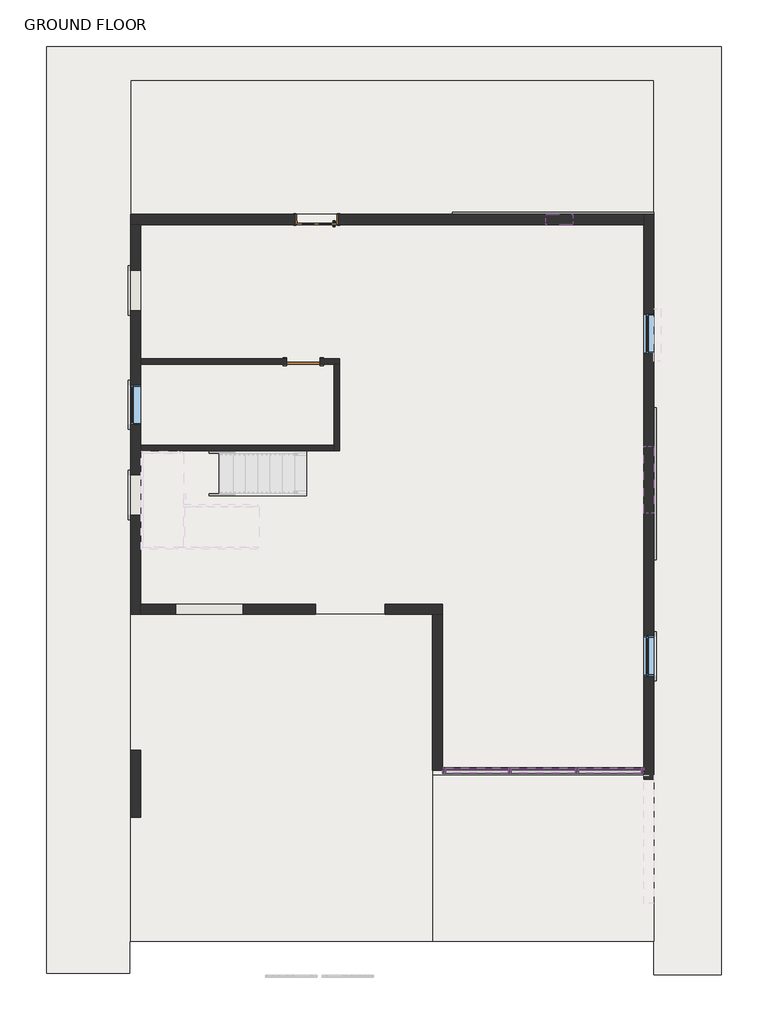
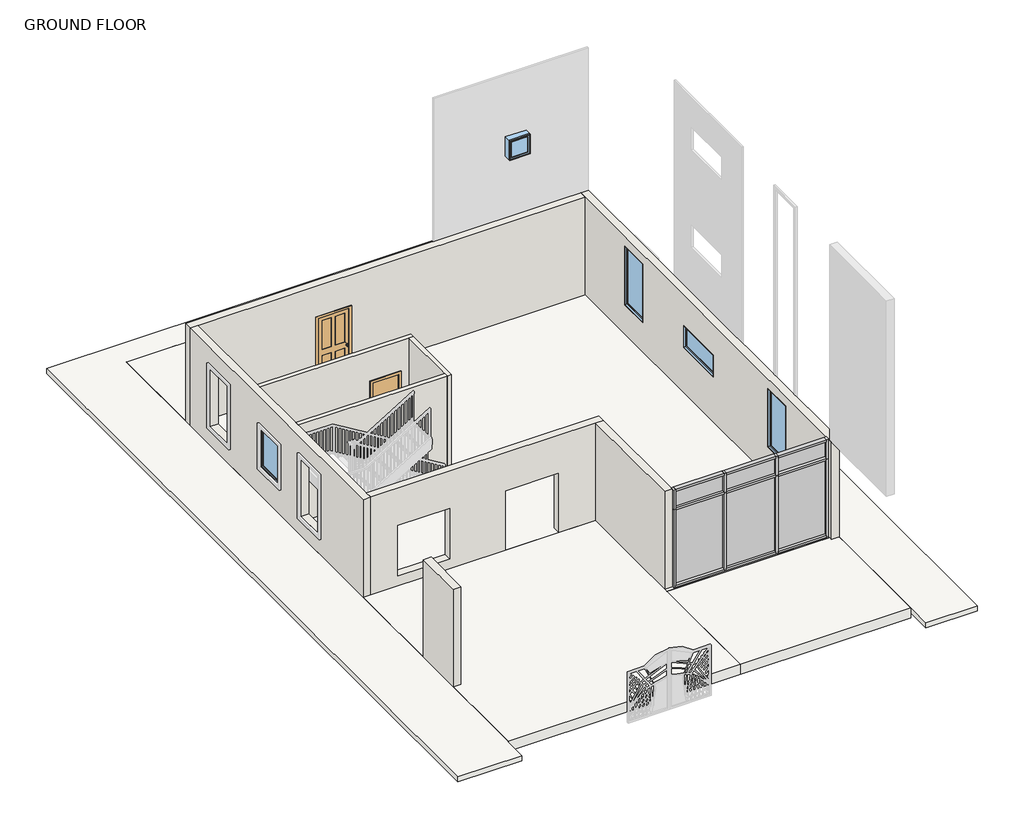
# One storey, part 1 of 3: 17 members, 9 walls, 6 plates, 5 slabs, 5 windows, 2 doors.
"""IFC4 building model written with IfcOpenShell, lengths in millimetres."""

from ifc_helpers import new_model, si_unit, frame, origin, origin_with_axes, place, context, project, spatial, polyline, outline, extrude, faceted_brep, transform, mapped, element, save
from components import door_8a5afc22, door_1fe7f57d, member_f0fea5a5, member_ee409385, member_3473b942, member_19b327e1, member_2e265c97, member_a95d9ad3, member_6e77e263, member_47bfaf8a, system_panel_glazed_f9f53b74, system_panel_glazed_d986c6a7, system_panel_glazed_28169b10, system_panel_glazed_6dc8f8fc, window_80340324, window_c1f32544, window_2e8ca8a3, window_e88f44c6

model = new_model("IFC4")

# Units and contexts
model_context = context("Model", 3, world=origin())
ifc_project = project(units=[si_unit("LENGTHUNIT", "METRE", prefix="MILLI")], contexts=[model_context])

# Site, building, storey
site = spatial("IfcSite", under=ifc_project)
building = spatial("IfcBuilding", under=site)
storey = spatial("IfcBuildingStorey", under=building, Name="GROUND FLOOR", Elevation=304.8)

# Doors
placement = place(None, origin())
door_shape = door_8a5afc22(model_context)
element("IfcDoor", 1, ObjectType="Door-Interior-Single-4_Panel-Wood : 36\" x 80\"", at=placement, inside=storey, context=model_context, shape_type="MappedRepresentation", body=[
    mapped(door_shape, transform((-5763.4781265, 8218.7107468, 304.8), x_axis=(-1.0, 0.0, 0.0), y_axis=(0.0, -1.0, 0.0), z_axis=(0.0, 0.0, 1.0))),
])
door_2_shape = door_1fe7f57d(model_context)
element("IfcDoor", 2, ObjectType="Single-Flush : 30\" x 80\"", at=placement, inside=storey, context=model_context, shape_type="MappedRepresentation", body=[
    mapped(door_2_shape, transform((-6068.2781265, 4996.0857468, 304.8), x_axis=(-1.0, 0.0, 0.0), y_axis=(0.0, -1.0, 0.0), z_axis=(0.0, 0.0, 1.0))),
])

# Members
member_shape = member_f0fea5a5(model_context)
element("IfcMember", 3, ObjectType="Rectangular Mullion : 2.5\" x 5\" rectangular", at=placement, inside=storey, context=model_context, shape_type="MappedRepresentation", body=[
    mapped(member_shape, transform((-1381.9781264, -4274.9142532, 304.8), x_axis=(1.0, 0.0, 0.0), y_axis=(0.0, -1.0, 0.0), z_axis=(0.0, 0.0, -1.0))),
])
element("IfcMember", 4, ObjectType="Rectangular Mullion : 2.5\" x 5\" rectangular", at=placement, inside=storey, context=model_context, shape_type="MappedRepresentation", body=[
    mapped(member_shape, transform((142.0218734, -4274.9142532, 304.8), x_axis=(1.0, 0.0, 0.0), y_axis=(0.0, -1.0, 0.0), z_axis=(0.0, 0.0, -1.0))),
])
member_2_shape = member_ee409385(model_context)
element("IfcMember", 5, ObjectType="Rectangular Mullion : 2.5\" x 5\" rectangular", at=placement, inside=storey, context=model_context, shape_type="MappedRepresentation", body=[
    mapped(member_2_shape, transform((1666.0218735, -4274.9142532, 304.8), x_axis=(1.0, 0.0, 0.0), y_axis=(0.0, -1.0, 0.0), z_axis=(0.0, 0.0, -1.0))),
])
element("IfcMember", 6, ObjectType="Rectangular Mullion : 2.5\" x 5\" rectangular", at=placement, inside=storey, context=model_context, shape_type="MappedRepresentation", body=[
    mapped(member_2_shape, transform((-2905.9781265, -4274.9142532, 2743.2), x_axis=(-1.0, 0.0, 0.0), y_axis=(0.0, -1.0, 0.0), z_axis=(0.0, 0.0, 1.0))),
])
member_3_shape = member_3473b942(model_context)
element("IfcMember", 7, ObjectType="Rectangular Mullion : 2.5\" x 5\" rectangular", at=placement, inside=storey, context=model_context, shape_type="MappedRepresentation", body=[
    mapped(member_3_shape, transform((1602.5218735, -4274.9142532, 3352.8), x_axis=(0.0, 0.0, 1.0), y_axis=(0.0, -1.0, 0.0), z_axis=(1.0, 0.0, 0.0))),
])
element("IfcMember", 8, ObjectType="Rectangular Mullion : 2.5\" x 5\" rectangular", at=placement, inside=storey, context=model_context, shape_type="MappedRepresentation", body=[
    mapped(member_3_shape, transform((-1413.7281264, -4274.9142532, 3352.8), x_axis=(0.0, 0.0, 1.0), y_axis=(0.0, -1.0, 0.0), z_axis=(1.0, 0.0, 0.0))),
])
element("IfcMember", 9, ObjectType="Rectangular Mullion : 2.5\" x 5\" rectangular", at=placement, inside=storey, context=model_context, shape_type="MappedRepresentation", body=[
    mapped(member_3_shape, transform((-2842.4781265, -4274.9142532, 304.8), x_axis=(0.0, 0.0, -1.0), y_axis=(0.0, -1.0, 0.0), z_axis=(-1.0, 0.0, 0.0))),
])
element("IfcMember", 10, ObjectType="Rectangular Mullion : 2.5\" x 5\" rectangular", at=placement, inside=storey, context=model_context, shape_type="MappedRepresentation", body=[
    mapped(member_3_shape, transform((173.7718734, -4274.9142532, 304.8), x_axis=(0.0, 0.0, -1.0), y_axis=(0.0, -1.0, 0.0), z_axis=(-1.0, 0.0, 0.0))),
])
member_4_shape = member_19b327e1(model_context)
element("IfcMember", 11, ObjectType="Rectangular Mullion : 2.5\" x 5\" rectangular", at=placement, inside=storey, context=model_context, shape_type="MappedRepresentation", body=[
    mapped(member_4_shape, transform((110.2718734, -4274.9142532, 3352.8), x_axis=(0.0, 0.0, 1.0), y_axis=(0.0, -1.0, 0.0), z_axis=(1.0, 0.0, 0.0))),
])
element("IfcMember", 12, ObjectType="Rectangular Mullion : 2.5\" x 5\" rectangular", at=placement, inside=storey, context=model_context, shape_type="MappedRepresentation", body=[
    mapped(member_4_shape, transform((-1350.2281264, -4274.9142532, 304.8), x_axis=(0.0, 0.0, -1.0), y_axis=(0.0, -1.0, 0.0), z_axis=(-1.0, 0.0, 0.0))),
])
member_5_shape = member_2e265c97(model_context)
element("IfcMember", 13, ObjectType="Rectangular Mullion : 2.5\" x 5\" rectangular", at=placement, inside=storey, context=model_context, shape_type="MappedRepresentation", body=[
    mapped(member_5_shape, transform((-1413.7281264, -4274.9142532, 2743.2), x_axis=(0.0, 0.0, 1.0), y_axis=(0.0, -1.0, 0.0), z_axis=(1.0, 0.0, 0.0))),
])
element("IfcMember", 14, ObjectType="Rectangular Mullion : 2.5\" x 5\" rectangular", at=placement, inside=storey, context=model_context, shape_type="MappedRepresentation", body=[
    mapped(member_5_shape, transform((1602.5218735, -4274.9142532, 2743.2), x_axis=(0.0, 0.0, 1.0), y_axis=(0.0, -1.0, 0.0), z_axis=(1.0, 0.0, 0.0))),
])
member_6_shape = member_a95d9ad3(model_context)
element("IfcMember", 15, ObjectType="Rectangular Mullion : 2.5\" x 5\" rectangular", at=placement, inside=storey, context=model_context, shape_type="MappedRepresentation", body=[
    mapped(member_6_shape, transform((110.2718734, -4274.9142532, 2743.2), x_axis=(0.0, 0.0, 1.0), y_axis=(0.0, -1.0, 0.0), z_axis=(1.0, 0.0, 0.0))),
])
member_7_shape = member_6e77e263(model_context)
element("IfcMember", 16, ObjectType="Rectangular Mullion : 2.5\" x 5\" rectangular", at=placement, inside=storey, context=model_context, shape_type="MappedRepresentation", body=[
    mapped(member_7_shape, transform((-1381.9781264, -4274.9142532, 2743.2), x_axis=(1.0, 0.0, 0.0), y_axis=(0.0, -1.0, 0.0), z_axis=(0.0, 0.0, -1.0))),
])
element("IfcMember", 17, ObjectType="Rectangular Mullion : 2.5\" x 5\" rectangular", at=placement, inside=storey, context=model_context, shape_type="MappedRepresentation", body=[
    mapped(member_7_shape, transform((142.0218734, -4274.9142532, 2743.2), x_axis=(1.0, 0.0, 0.0), y_axis=(0.0, -1.0, 0.0), z_axis=(0.0, 0.0, -1.0))),
])
member_8_shape = member_47bfaf8a(model_context)
element("IfcMember", 18, ObjectType="Rectangular Mullion : 2.5\" x 5\" rectangular", at=placement, inside=storey, context=model_context, shape_type="MappedRepresentation", body=[
    mapped(member_8_shape, transform((-2905.9781265, -4274.9142532, 3352.8), x_axis=(-1.0, 0.0, 0.0), y_axis=(0.0, -1.0, 0.0), z_axis=(0.0, 0.0, 1.0))),
])
element("IfcMember", 19, ObjectType="Rectangular Mullion : 2.5\" x 5\" rectangular", at=placement, inside=storey, context=model_context, shape_type="MappedRepresentation", body=[
    mapped(member_8_shape, transform((1666.0218735, -4274.9142532, 2743.2), x_axis=(1.0, 0.0, 0.0), y_axis=(0.0, -1.0, 0.0), z_axis=(0.0, 0.0, -1.0))),
])

# Plates
system_panel_glazed_shape = system_panel_glazed_f9f53b74(model_context)
element("IfcPlate", 20, ObjectType="System Panel : Glazed", at=placement, inside=storey, context=model_context, shape_type="MappedRepresentation", body=[
    mapped(system_panel_glazed_shape, transform((-2128.1031264, -4274.9142532, 368.3), x_axis=(1.0, 0.0, 0.0), y_axis=(0.0, 1.0, 0.0), z_axis=(0.0, 0.0, 1.0))),
])
element("IfcPlate", 21, ObjectType="System Panel : Glazed", at=placement, inside=storey, context=model_context, shape_type="MappedRepresentation", body=[
    mapped(system_panel_glazed_shape, transform((888.1468735, -4274.9142532, 368.3), x_axis=(1.0, 0.0, 0.0), y_axis=(0.0, 1.0, 0.0), z_axis=(0.0, 0.0, 1.0))),
])
system_panel_glazed_2_shape = system_panel_glazed_d986c6a7(model_context)
element("IfcPlate", 22, ObjectType="System Panel : Glazed", at=placement, inside=storey, context=model_context, shape_type="MappedRepresentation", body=[
    mapped(system_panel_glazed_2_shape, transform((-619.9781265, -4274.9142532, 368.3), x_axis=(1.0, 0.0, 0.0), y_axis=(0.0, 1.0, 0.0), z_axis=(0.0, 0.0, 1.0))),
])
system_panel_glazed_3_shape = system_panel_glazed_28169b10(model_context)
element("IfcPlate", 23, ObjectType="System Panel : Glazed", at=placement, inside=storey, context=model_context, shape_type="MappedRepresentation", body=[
    mapped(system_panel_glazed_3_shape, transform((-2128.1031264, -4274.9142532, 2774.95), x_axis=(1.0, 0.0, 0.0), y_axis=(0.0, 1.0, 0.0), z_axis=(0.0, 0.0, 1.0))),
])
element("IfcPlate", 24, ObjectType="System Panel : Glazed", at=placement, inside=storey, context=model_context, shape_type="MappedRepresentation", body=[
    mapped(system_panel_glazed_3_shape, transform((888.1468735, -4274.9142532, 2774.95), x_axis=(1.0, 0.0, 0.0), y_axis=(0.0, 1.0, 0.0), z_axis=(0.0, 0.0, 1.0))),
])
system_panel_glazed_4_shape = system_panel_glazed_6dc8f8fc(model_context)
element("IfcPlate", 25, ObjectType="System Panel : Glazed", at=placement, inside=storey, context=model_context, shape_type="MappedRepresentation", body=[
    mapped(system_panel_glazed_4_shape, transform((-619.9781265, -4274.9142532, 2774.95), x_axis=(1.0, 0.0, 0.0), y_axis=(0.0, 1.0, 0.0), z_axis=(0.0, 0.0, 1.0))),
])

# Slabs
element("IfcSlab", 26, at=placement, inside=storey, context=model_context, shape_type="SweptSolid", body=[
    extrude(outline(polyline([(-3134.5781265, -731.6142532), (-3134.5781265, -8147.8779205), (-9992.5781265, -8147.8779205), (-9992.5781265, -731.6142532), (-3134.5781265, -731.6142532)])), origin_with_axes(), (0.0, 0.0, 1.0), 304.8),
])
element("IfcSlab", 27, at=placement, inside=storey, context=model_context, shape_type="SweptSolid", body=[
    extrude(outline(polyline([(1894.6218735, -4389.2142532), (1894.6218735, -8147.9432518), (-3134.5781265, -8147.9432518), (-3134.5781265, -4389.2142532), (1894.6218735, -4389.2142532)])), origin_with_axes(), (0.0, 0.0, 1.0), 304.8),
])
element("IfcSlab", 28, at=placement, inside=storey, context=model_context, shape_type="SweptSolid", body=[
    extrude(outline(polyline([(1894.6218735, 8336.1857468), (-9992.5781265, 8336.1857468), (-9992.5781265, 11384.1857468), (1894.6218735, 11384.1857468), (1894.6218735, 8336.1857468)])), origin_with_axes(), (0.0, 0.0, 1.0), 304.8),
])
element("IfcSlab", 29, ObjectType="marble flooring 1'", at=placement, inside=storey, context=model_context, shape_type="SweptSolid", body=[
    extrude(outline(polyline([(-9992.5781265, 8336.1857468), (1894.6218735, 8336.1857468), (1894.6218735, -4389.2142532), (-3134.5781265, -4389.2142532), (-3134.5781265, -731.6142532), (-9992.5781265, -731.6142532), (-9992.5781265, 8336.1857468)])), origin_with_axes(), (0.0, 0.0, 1.0), 304.8),
])
element("IfcSlab", 30, ObjectType="outside flooring 6\"", at=placement, inside=storey, context=model_context, shape_type="SweptSolid", body=[
    extrude(outline(polyline([(3418.6218735, 12146.1857468), (3418.6218735, -8909.9432518), (1894.6218735, -8909.9432518), (1894.6218735, -8147.9432518), (1894.6218735, 11384.1857468), (-9992.5781265, 11384.1857468), (-9992.5781265, -8147.9432518), (-10006.8176097, -8147.9432518), (-10006.8176097, -8878.1279205), (-11897.5781265, -8878.1279205), (-11897.5781265, 12146.1857468), (3418.6218735, 12146.1857468)])), frame((0.0, 0.0, 152.4), z_axis=(0.0, 0.0, 1.0), x_axis=(1.0, 0.0, 0.0)), (0.0, 0.0, 1.0), 152.4),
])

# Walls
element("IfcWall", 31, ObjectType="Generic - 5\"", at=placement, inside=storey, context=model_context, shape_type="Brep", body=[
    faceted_brep([(-9763.9781265, 4932.5857468, 304.8), (-6449.2781265, 4932.5857468, 304.8), (-6449.2781265, 4932.5857468, 2336.8), (-5687.2781265, 4932.5857468, 2336.8), (-5687.2781265, 4932.5857468, 304.8), (-5369.7781265, 4932.5857468, 304.8), (-5242.7781265, 4932.5857468, 304.8), (-5242.7781265, 4932.5857468, 3352.8), (-5369.7781265, 4932.5857468, 3352.8), (-9763.9781265, 4932.5857468, 3352.8), (-6449.2781265, 5059.5857468, 2336.8), (-6449.2781265, 5059.5857468, 304.8), (-9763.9781265, 5059.5857468, 304.8), (-9763.9781265, 5059.5857468, 3352.8), (-5242.7781265, 5059.5857468, 3352.8), (-5242.7781265, 5059.5857468, 304.8), (-5687.2781265, 5059.5857468, 304.8), (-5687.2781265, 5059.5857468, 2336.8)], [[[0, 1, 2, 3, 4, 5, 6, 7, 8, 9]], [[10, 11, 12, 13, 14, 15, 16, 17]], [[16, 15, 6, 5, 4]], [[12, 11, 1, 0]], [[9, 8, 7, 14, 13]], [[0, 9, 13, 12]], [[7, 6, 15, 14]], [[2, 1, 11, 10]], [[3, 2, 10, 17]], [[4, 3, 17, 16]]]),
])
element("IfcWall", 32, ObjectType="Generic - 5\"", at=placement, inside=storey, context=model_context, shape_type="Brep", body=[
    faceted_brep([(-5369.7781265, 4932.5857468, 304.8), (-5369.7781265, 3103.7857468, 304.8), (-5369.7781265, 2976.7857468, 304.8), (-5369.7781265, 2976.7857468, 3352.8), (-5369.7781265, 3103.7857468, 3352.8), (-5369.7781265, 4932.5857468, 3352.8), (-5242.7781265, 4932.5857468, 304.8), (-5242.7781265, 4932.5857468, 3352.8), (-5242.7781265, 2976.7857468, 3352.8), (-5242.7781265, 2976.7857468, 304.8)], [[[0, 1, 2, 3, 4, 5]], [[6, 7, 8, 9]], [[2, 1, 0, 6, 9]], [[5, 4, 3, 8, 7]], [[0, 5, 7, 6]], [[3, 2, 9, 8]]]),
])
element("IfcWall", 33, ObjectType="Generic - 5\"", at=placement, inside=storey, context=model_context, shape_type="SweptSolid", body=[
    extrude(outline(polyline([(-9763.9781265, 3103.7857468), (-5369.7781265, 3103.7857468), (-5369.7781265, 2976.7857468), (-9763.9781265, 2976.7857468), (-9763.9781265, 3103.7857468)])), frame((0.0, 0.0, 304.8), z_axis=(0.0, 0.0, 1.0), x_axis=(1.0, 0.0, 0.0)), (0.0, 0.0, 1.0), 3048.0),
])
element("IfcWall", 34, ObjectType="OUTER WALL THICKNESS 9\"", at=placement, inside=storey, context=model_context, shape_type="Brep", body=[
    faceted_brep([(1894.6218735, -4478.1142532, 304.8), (1894.6218735, 8336.1857468, 304.8), (1894.6218735, 8336.1857468, 3352.8), (1894.6218735, -4478.1142532, 3352.8), (1894.6218735, -1226.9142532, 3048.0), (1894.6218735, -1226.9142532, 1219.2), (1894.6218735, -2141.3142532, 1219.2), (1894.6218735, -2141.3142532, 3048.0), (1894.6218735, 6088.2857468, 3048.0), (1894.6218735, 6088.2857468, 1219.2), (1894.6218735, 5173.8857468, 1219.2), (1894.6218735, 5173.8857468, 3048.0), (1894.6218735, 3078.0165128, 2400.2767967), (1894.6218735, 3078.0165128, 1714.4767967), (1894.6218735, 1554.0165128, 1714.4767967), (1894.6218735, 1554.0165128, 2400.2767967), (1666.0218735, -4478.1142532, 304.8), (1666.0218735, -4478.1142532, 3352.8), (1666.0218735, 8107.5857468, 3352.8), (1666.0218735, 8336.1857468, 3352.8), (1666.0218735, 8336.1857468, 304.8), (1666.0218735, 8107.5857468, 304.8), (1666.0218735, -1226.9142532, 3048.0), (1666.0218735, -2141.3142532, 3048.0), (1666.0218735, -2141.3142532, 1219.2), (1666.0218735, -1226.9142532, 1219.2), (1666.0218735, 6088.2857468, 3048.0), (1666.0218735, 5173.8857468, 3048.0), (1666.0218735, 5173.8857468, 1219.2), (1666.0218735, 6088.2857468, 1219.2), (1666.0218735, 3078.0165128, 2400.2767967), (1666.0218735, 1554.0165128, 2400.2767967), (1666.0218735, 1554.0165128, 1714.4767967), (1666.0218735, 3078.0165128, 1714.4767967)], [[[0, 1, 2, 3], [4, 5, 6, 7], [8, 9, 10, 11], [12, 13, 14, 15]], [[16, 17, 18, 19, 20, 21], [22, 23, 24, 25], [26, 27, 28, 29], [30, 31, 32, 33]], [[1, 0, 16, 21, 20]], [[3, 2, 19, 18, 17]], [[0, 3, 17, 16]], [[2, 1, 20, 19]], [[5, 4, 22, 25]], [[6, 5, 25, 24]], [[7, 6, 24, 23]], [[4, 7, 23, 22]], [[9, 8, 26, 29]], [[10, 9, 29, 28]], [[11, 10, 28, 27]], [[8, 11, 27, 26]], [[13, 12, 30, 33]], [[14, 13, 33, 32]], [[15, 14, 32, 31]], [[12, 15, 31, 30]]]),
])
element("IfcWall", 35, ObjectType="OUTER WALL THICKNESS 9\"", at=placement, inside=storey, context=model_context, shape_type="Brep", body=[
    faceted_brep([(-9992.5781265, 8336.1857468, 3352.8), (1666.0218735, 8336.1857468, 3352.8), (1666.0218735, 8336.1857468, 304.8), (-5280.8781265, 8336.1857468, 304.8), (-5280.8781265, 8336.1857468, 2362.2), (-6246.0781265, 8336.1857468, 2362.2), (-6246.0781265, 8336.1857468, 304.8), (-9992.5781265, 8336.1857468, 304.8), (1666.0218735, 8107.5857468, 3352.8), (-9763.9781265, 8107.5857468, 3352.8), (-9992.5781265, 8107.5857468, 3352.8), (-9992.5781265, 8107.5857468, 304.8), (-9763.9781265, 8107.5857468, 304.8), (-6246.0781265, 8107.5857468, 304.8), (-6246.0781265, 8107.5857468, 2362.2), (-5280.8781265, 8107.5857468, 2362.2), (-5280.8781265, 8107.5857468, 304.8), (1666.0218735, 8107.5857468, 304.8)], [[[0, 1, 2, 3, 4, 5, 6, 7]], [[8, 9, 10, 11, 12, 13, 14, 15, 16, 17]], [[2, 17, 16, 3]], [[11, 7, 6, 13, 12]], [[1, 0, 10, 9, 8]], [[2, 1, 8, 17]], [[0, 7, 11, 10]], [[5, 14, 13, 6]], [[14, 5, 4, 15]], [[15, 4, 3, 16]]]),
])
element("IfcWall", 36, ObjectType="OUTER WALL THICKNESS 9\"", at=placement, inside=storey, context=model_context, shape_type="Brep", body=[
    faceted_brep([(-9992.5781265, 8107.5857468, 304.8), (-9992.5781265, -731.6142532, 304.8), (-9992.5781265, -731.6142532, 3352.8), (-9992.5781265, 8107.5857468, 3352.8), (-9992.5781265, 4475.3857468, 2438.4), (-9992.5781265, 3560.9857468, 2438.4), (-9992.5781265, 3560.9857468, 1219.2), (-9992.5781265, 4475.3857468, 1219.2), (-9992.5781265, 7066.1857468, 2743.2), (-9992.5781265, 6151.7857468, 2743.2), (-9992.5781265, 6151.7857468, 914.4), (-9992.5781265, 7066.1857468, 914.4), (-9992.5781265, 2430.6857468, 2743.2), (-9992.5781265, 1516.2857468, 2743.2), (-9992.5781265, 1516.2857468, 914.4), (-9992.5781265, 2430.6857468, 914.4), (-9763.9781265, 8107.5857468, 304.8), (-9763.9781265, 8107.5857468, 3352.8), (-9763.9781265, 5059.5857468, 3352.8), (-9763.9781265, 4932.5857468, 3352.8), (-9763.9781265, 3103.7857468, 3352.8), (-9763.9781265, 2976.7857468, 3352.8), (-9763.9781265, -503.0142532, 3352.8), (-9763.9781265, -731.6142532, 3352.8), (-9763.9781265, -731.6142532, 304.8), (-9763.9781265, -503.0142532, 304.8), (-9763.9781265, 2976.7857468, 304.8), (-9763.9781265, 3103.7857468, 304.8), (-9763.9781265, 4932.5857468, 304.8), (-9763.9781265, 5059.5857468, 304.8), (-9763.9781265, 4475.3857468, 2438.4), (-9763.9781265, 4475.3857468, 1219.2), (-9763.9781265, 3560.9857468, 1219.2), (-9763.9781265, 3560.9857468, 2438.4), (-9763.9781265, 7066.1857468, 2743.2), (-9763.9781265, 7066.1857468, 914.4), (-9763.9781265, 6151.7857468, 914.4), (-9763.9781265, 6151.7857468, 2743.2), (-9763.9781265, 2430.6857468, 2743.2), (-9763.9781265, 2430.6857468, 914.4), (-9763.9781265, 1516.2857468, 914.4), (-9763.9781265, 1516.2857468, 2743.2)], [[[0, 1, 2, 3], [4, 5, 6, 7], [8, 9, 10, 11], [12, 13, 14, 15]], [[16, 17, 18, 19, 20, 21, 22, 23, 24, 25, 26, 27, 28, 29], [30, 31, 32, 33], [34, 35, 36, 37], [38, 39, 40, 41]], [[1, 0, 16, 29, 28, 27, 26, 25, 24]], [[3, 2, 23, 22, 21, 20, 19, 18, 17]], [[0, 3, 17, 16]], [[2, 1, 24, 23]], [[31, 30, 4, 7]], [[32, 31, 7, 6]], [[33, 32, 6, 5]], [[30, 33, 5, 4]], [[35, 34, 8, 11]], [[36, 35, 11, 10]], [[37, 36, 10, 9]], [[34, 37, 9, 8]], [[39, 38, 12, 15]], [[40, 39, 15, 14]], [[41, 40, 14, 13]], [[38, 41, 13, 12]]]),
])
element("IfcWall", 37, ObjectType="OUTER WALL THICKNESS 9\"", at=placement, inside=storey, context=model_context, shape_type="Brep", body=[
    faceted_brep([(-2905.9781265, -731.6142532, 3352.8), (-3134.5781265, -731.6142532, 3352.8), (-9763.9781265, -731.6142532, 3352.8), (-9763.9781265, -731.6142532, 304.8), (-5788.8781265, -731.6142532, 304.8), (-5788.8781265, -731.6142532, 2159.0), (-4214.0781265, -731.6142532, 2159.0), (-4214.0781265, -731.6142532, 304.8), (-3134.5781265, -731.6142532, 304.8), (-2905.9781265, -731.6142532, 304.8), (-8963.8781265, -731.6142532, 2184.4), (-7439.8781265, -731.6142532, 2184.4), (-7439.8781265, -731.6142532, 609.6), (-8963.8781265, -731.6142532, 609.6), (-9763.9781265, -503.0142532, 3352.8), (-2905.9781265, -503.0142532, 3352.8), (-2905.9781265, -503.0142532, 304.8), (-4214.0781265, -503.0142532, 304.8), (-4214.0781265, -503.0142532, 2159.0), (-5788.8781265, -503.0142532, 2159.0), (-5788.8781265, -503.0142532, 304.8), (-9763.9781265, -503.0142532, 304.8), (-8963.8781265, -503.0142532, 2184.4), (-8963.8781265, -503.0142532, 609.6), (-7439.8781265, -503.0142532, 609.6), (-7439.8781265, -503.0142532, 2184.4)], [[[0, 1, 2, 3, 4, 5, 6, 7, 8, 9], [10, 11, 12, 13]], [[14, 15, 16, 17, 18, 19, 20, 21], [22, 23, 24, 25]], [[3, 21, 20, 4]], [[16, 9, 8, 7, 17]], [[2, 1, 0, 15, 14]], [[3, 2, 14, 21]], [[0, 9, 16, 15]], [[19, 5, 4, 20]], [[5, 19, 18, 6]], [[6, 18, 17, 7]], [[23, 22, 10, 13]], [[24, 23, 13, 12]], [[25, 24, 12, 11]], [[22, 25, 11, 10]]]),
])
element("IfcWall", 38, ObjectType="OUTER WALL THICKNESS 9\"", at=placement, inside=storey, context=model_context, shape_type="SweptSolid", body=[
    extrude(outline(polyline([(-3134.5781265, -4274.9142532), (-3134.5781265, -731.6142532), (-2905.9781265, -731.6142532), (-2905.9781265, -4274.9142532), (-3134.5781265, -4274.9142532)])), frame((0.0, 0.0, 304.8), z_axis=(0.0, 0.0, 1.0), x_axis=(1.0, 0.0, 0.0)), (0.0, 0.0, 1.0), 3048.0),
])
element("IfcWall", 39, ObjectType="OUTER WALL THICKNESS 9\"", at=placement, inside=storey, context=model_context, shape_type="SweptSolid", body=[
    extrude(outline(polyline([(-9992.5781265, -5341.7142532), (-9992.5781265, -3817.7142532), (-9763.9781265, -3817.7142532), (-9763.9781265, -5341.7142532), (-9992.5781265, -5341.7142532)])), frame((0.0, 0.0, 304.8), z_axis=(0.0, 0.0, 1.0), x_axis=(1.0, 0.0, 0.0)), (0.0, 0.0, 1.0), 3048.0),
])

# Windows
window_shape = window_80340324(model_context)
element("IfcWindow", 40, ObjectType="Fixed : 24\" x 24\"", at=placement, inside=storey, context=model_context, shape_type="MappedRepresentation", body=[
    mapped(window_shape, transform((-289.7781265, 8221.8857468, 4358.0336242), x_axis=(-1.0, 0.0, 0.0), y_axis=(0.0, -1.0, 0.0), z_axis=(0.0, 0.0, 1.0))),
])
window_2_shape = window_c1f32544(model_context)
element("IfcWindow", 41, ObjectType="Fixed : 36\" x 48\"", at=placement, inside=storey, context=model_context, shape_type="MappedRepresentation", body=[
    mapped(window_2_shape, transform((-9878.2781265, 4056.2857468, 304.8), x_axis=(0.0, 1.0, 0.0), y_axis=(-1.0, 0.0, 0.0), z_axis=(0.0, 0.0, 1.0))),
])
window_3_shape = window_2e8ca8a3(model_context)
element("IfcWindow", 42, ObjectType="Fixed : window 3' x 6\"", at=placement, inside=storey, context=model_context, shape_type="MappedRepresentation", body=[
    mapped(window_3_shape, transform((1780.3218735, -1646.0142532, 304.8), x_axis=(0.0, 1.0, 0.0), y_axis=(-1.0, 0.0, 0.0), z_axis=(0.0, 0.0, 1.0))),
])
element("IfcWindow", 43, ObjectType="Fixed : window 3' x 6\"", at=placement, inside=storey, context=model_context, shape_type="MappedRepresentation", body=[
    mapped(window_3_shape, transform((1780.3218735, 5669.1857468, 304.8), x_axis=(0.0, 1.0, 0.0), y_axis=(-1.0, 0.0, 0.0), z_axis=(0.0, 0.0, 1.0))),
])
window_4_shape = window_e88f44c6(model_context)
element("IfcWindow", 44, ObjectType="Fixed : window length 5' x 2'3\"", at=placement, inside=storey, context=model_context, shape_type="MappedRepresentation", body=[
    mapped(window_4_shape, transform((1780.3218735, 2354.1165128, 800.0767967), x_axis=(0.0, 1.0, 0.0), y_axis=(-1.0, 0.0, 0.0), z_axis=(0.0, 0.0, 1.0))),
])

save(model, "model.ifc")

# Revit data of these elements
# Type "Door-Interior-Single-4_Panel-Wood : 36\" x 80\""
#   Type Mark = "9"
#   Assembly Code = "C1020300"
#   Analytic Construction = "Wooden"
#   Top Rail = 0' - 4 11/16"
#   Thickness = 0' - 1 3/8"
#   Thermal Resistance (R) = 2.5876 (h·ft²·°F)/BTU
#   Swing Angle [instance default] = 90.00°
#   Stiles = 0' - 4 3/4"
#   Rough Width = 3' - 2"
#   Rough Height = 6' - 9"
#   Mullion = 0' - 4 1/2"
#   Lock Rail = 0' - 7 1/2"
#   Height = 6' - 8"
#   Width = 3' - 0"
#   Heat Transfer Coefficient (U) = 0.3865 BTU/(h·ft²·°F)
#   Bottom Rail = 0' - 9 1/8"
#   Trim Material = Cherry
#   Panel Material = Cherry
#   Frame Material = Cherry
#   Door Handle Material = Aluminum
#   Visual Light Transmittance = 0
#   Solar Heat Gain Coefficient = 0
#   Wall Closure = (empty or 0)
#   Function = (empty or 0)
# Type "Single-Flush : 30\" x 80\""
#   Type Mark = "5"
#   Construction Type Id = "MDOOR"
#   Assembly Code = "C1020"
#   Analytic Construction = "Metal"
#   Thickness = 0' - 2"
#   Heat Transfer Coefficient (U) = 0.651978 BTU/(h·ft²·°F)
#   Height = 6' - 8"
#   Trim Projection Ext = 0' - 1"
#   Trim Projection Int = 0' - 1"
#   Trim Width = 0' - 3"
#   Width = 2' - 6"
#   Define Thermal Properties by = 1
#   Define Thermal Properties by = 1
#   Door Material = Door - Panel
#   Frame Material = Door - Frame
#   Visual Light Transmittance = 0
#   Solar Heat Gain Coefficient = 0
#   Function = (empty or 0)
#   Wall Closure = (empty or 0)
# Type "Rectangular Mullion : 2.5\" x 5\" rectangular"
#   built-in parameter 1007304 = 0.416667 (stored number, unit not read)
#   built-in parameter 1007301 = 0.104167 (stored number, unit not read)
#   built-in parameter 1007300 = 0.104167 (stored number, unit not read)
# Type "System Panel : Glazed"
#   Construction Type Id = "GSP4R"
#   Analytic Construction = "1/8 in Pilkington single glazing"
#   Visual Light Transmittance = 0.9
#   Solar Heat Gain Coefficient = 0.86
#   Heat Transfer Coefficient (U) = 1.18115 BTU/(h·ft²·°F)
#   Define Thermal Properties by = 1
# Type
#   Assembly Code = "B1010"
#   Function = 0
# Type "marble flooring 1'"
#   Assembly Code = "B1010"
#   Function = 0
#   Layers, outside or top first: 1' - 0" "MARBLE FLOORING" (function 1)
# Type "outside flooring 6\""
#   Assembly Code = "B1010"
#   Function = 0
# Type "Generic - 5\""
#   Assembly Code = "B2010"
#   Layers, outside or top first: 0' - 5" no material (function 1)
# Type "OUTER WALL THICKNESS 9\""
#   Assembly Code = "B2010"
#   Layers, outside or top first: 0' - 9" "WALL PAINT" (function 1)
# Type "Fixed : 24\" x 24\""
#   Type Mark = "3"
#   Construction Type Id = "GSP4R"
#   Assembly Code = "B2020100"
#   Analytic Construction = "1/8 in Pilkington single glazing"
#   Visual Light Transmittance = 0.9
#   Solar Heat Gain Coefficient = 0.78
#   Heat Transfer Coefficient (U) = 0.6496 BTU/(h·ft²·°F)
#   Height = 2' - 0"
#   Default Sill Height = 3' - 0"
#   Width = 2' - 0"
#   Window Inset = 0' - 0 3/4"
#   Define Thermal Properties by = 1
#   Define Thermal Properties by = 1
#   Glass Pane Material = Glass
#   Sash Material = Sash
#   Wall Closure = (empty or 0)
# Type "Fixed : 36\" x 48\""
#   Type Mark = "1"
#   Construction Type Id = "GSP4R"
#   Assembly Code = "B2020100"
#   Analytic Construction = "1/8 in Pilkington single glazing"
#   Visual Light Transmittance = 0.9
#   Solar Heat Gain Coefficient = 0.78
#   Heat Transfer Coefficient (U) = 0.6496 BTU/(h·ft²·°F)
#   Height = 4' - 0"
#   Default Sill Height = 3' - 0"
#   Width = 3' - 0"
#   Window Inset = 0' - 0 3/4"
#   Define Thermal Properties by = 1
#   Define Thermal Properties by = 1
#   Glass Pane Material = Glass
#   Sash Material = Sash
#   Wall Closure = (empty or 0)
# Type "Fixed : window 3' x 6\""
#   Type Mark = "26"
#   Construction Type Id = "GSP4R"
#   Assembly Code = "B2020100"
#   Analytic Construction = "1/8 in Pilkington single glazing"
#   Visual Light Transmittance = 0.9
#   Solar Heat Gain Coefficient = 0.78
#   Heat Transfer Coefficient (U) = 0.6496 BTU/(h·ft²·°F)
#   Height = 6' - 0"
#   Default Sill Height = 3' - 0"
#   Width = 3' - 0"
#   Window Inset = 0' - 2"
#   Define Thermal Properties by = 1
#   Glass Pane Material = Glass
#   Sash Material = Sash
#   Wall Closure = (empty or 0)
# Type "Fixed : window length 5' x 2'3\""
#   Type Mark = "28"
#   Construction Type Id = "GSP4R"
#   Assembly Code = "B2020100"
#   Analytic Construction = "1/8 in Pilkington single glazing"
#   Visual Light Transmittance = 0.9
#   Solar Heat Gain Coefficient = 0.78
#   Heat Transfer Coefficient (U) = 0.6496 BTU/(h·ft²·°F)
#   Height = 2' - 3"
#   Default Sill Height = 3' - 0"
#   Width = 5' - 0"
#   Window Inset = 0' - 2"
#   Define Thermal Properties by = 1
#   Glass Pane Material = Glass
#   Sash Material = Sash
#   Wall Closure = (empty or 0)
# Element 1 (IfcDoor, "Door-Interior-Single-4_Panel-Wood : 36\" x 80\"")
#   Swing Angle = 90.00°
#   Phase Created = New Construction
#   Materials on its faces: "Cherry", "Aluminum"
# Element 2 (IfcDoor, "Single-Flush : 30\" x 80\"")
#   Phase Created = New Construction
#   Materials on its faces: "Door - Frame", "Door - Panel"
# Elements 3, 4, 5, 6, 7, 8, 9, 10, 11, 12, 13, 14, 15, 16, 17, 18, 19 (IfcMember, "Rectangular Mullion : 2.5\" x 5\" rectangular")
#   Phase Created = New Construction
#   Materials on its faces: "BLACK COLOUR"
# Elements 20, 21, 22, 23, 24, 25 (IfcPlate, "System Panel : Glazed")
#   Phase Created = New Construction
#   Materials on its faces: "Glass"
# Elements 26, 27, 28 (IfcSlab)
#   Height Offset From Level = 0' - 0"
#   Phase Created = New Construction
# Element 29 (IfcSlab, "marble flooring 1'")
#   built-in parameter 1001955 = 3.14159 (stored number, unit not read)
#   Height Offset From Level = 0' - 0"
#   Phase Created = New Construction
#   Materials on its faces: "MARBLE FLOORING"
# Element 30 (IfcSlab, "outside flooring 6\"")
#   Height Offset From Level = 0' - 0"
#   Phase Created = New Construction
# Elements 31, 32, 33 (IfcWall, "Generic - 5\"")
#   Top Offset = 0' - 0"
#   Base Offset = 0' - 0"
#   wall height = 10' - 0"
#   Phase Created = New Construction
#   Base Constraint = GROUND FLOOR
#   Top Constraint = FIRST FLOOR
#   Materials on its faces: "Default Wall"
# Elements 34, 35, 37, 38, 39 (IfcWall, "OUTER WALL THICKNESS 9\"")
#   Top Offset = 0' - 0"
#   Base Offset = 0' - 0"
#   Unconnected Height = 10' - 0"
#   wall height = 10' - 0"
#   Phase Created = New Construction
#   Base Constraint = GROUND FLOOR
#   Materials on its faces: "WALL PAINT"
# Element 36 (IfcWall, "OUTER WALL THICKNESS 9\"")
#   Top Offset = 0' - 0"
#   Base Offset = 0' - 0"
#   wall height = 10' - 0"
#   Phase Created = New Construction
#   Base Constraint = GROUND FLOOR
#   Top Constraint = FIRST FLOOR
#   Materials on its faces: "WALL PAINT"
# Element 40 (IfcWindow, "Fixed : 24\" x 24\"")
#   Mark = "27"
#   Phase Created = New Construction
#   Materials on its faces: "Sash", "Glass"
# Element 41 (IfcWindow, "Fixed : 36\" x 48\"")
#   Mark = "1"
#   Phase Created = New Construction
#   Materials on its faces: "Sash", "Glass"
# Element 42 (IfcWindow, "Fixed : window 3' x 6\"")
#   Mark = "5"
#   Phase Created = New Construction
#   Materials on its faces: "Sash", "Glass"
# Element 43 (IfcWindow, "Fixed : window 3' x 6\"")
#   Mark = "6"
#   Phase Created = New Construction
#   Materials on its faces: "Sash", "Glass"
# Element 44 (IfcWindow, "Fixed : window length 5' x 2'3\"")
#   Mark = "18"
#   Phase Created = New Construction
#   Materials on its faces: "Sash", "Glass"
# Materials
#   "Cherry": class "Wood", colour RGB 226 177 128, transparency 0, Description = "Prunus Serotina", Cost = 0
#   "Aluminum": class "Metal", colour RGB 247 247 247, transparency 0, Description = "Aluminum 6061", Cost = 0
#   "Door - Panel": class "Wood", colour RGB 210 159 95, transparency 0, Cost = 0
#   "Door - Frame": colour RGB 118 70 51, transparency 0, Cost = 0
#   "MARBLE FLOORING": class "Generic", colour RGB 120 120 120, transparency 0, Cost = 0
#   "WALL PAINT": class "Generic", colour RGB 120 120 120, transparency 0, Cost = 0
#   "Glass": class "Glass", colour RGB 0 128 192, transparency 0.75, Description = "Soda Lime Glass", Cost = 0
#   "Sash": class "Wood", colour RGB 224 178 126, transparency 0, Cost = 0
#   "BLACK COLOUR": class "Generic", colour RGB 120 120 120, transparency 0, Cost = 0
#   "Default Wall": colour RGB 128 128 128, transparency 0, Cost = 0
# Room at (-815.235, 4540.595) mm, phase "New Construction", upper level "GROUND FLOOR", upper offset 10' - 0", lower offset 0' - 0"
#   Number = "4"
#   Name = "LIVING AND DINING ROOM"
# Room at (-7592.278, 7034.011) mm, phase "New Construction", upper level "GROUND FLOOR", upper offset 10' - 0", lower offset 0' - 0"
#   Number = "5"
#   Name = "KITCHEN"
# Room, not placed, phase "New Construction", upper offset 0' - 0", lower offset 0' - 0"
#   Number = "6"
#   Name = "Room"
# Room at (-4048.978, 1973.486) mm, phase "New Construction", upper level "GROUND FLOOR", upper offset 10' - 0", lower offset 0' - 0"
#   Number = "2"
#   Name = "ENTRANCE PASSAGE"
# Room at (-7592.278, 4018.186) mm, phase "New Construction", upper level "GROUND FLOOR", upper offset 10' - 0", lower offset 0' - 0"
#   Number = "3"
#   Name = "TOILET"
